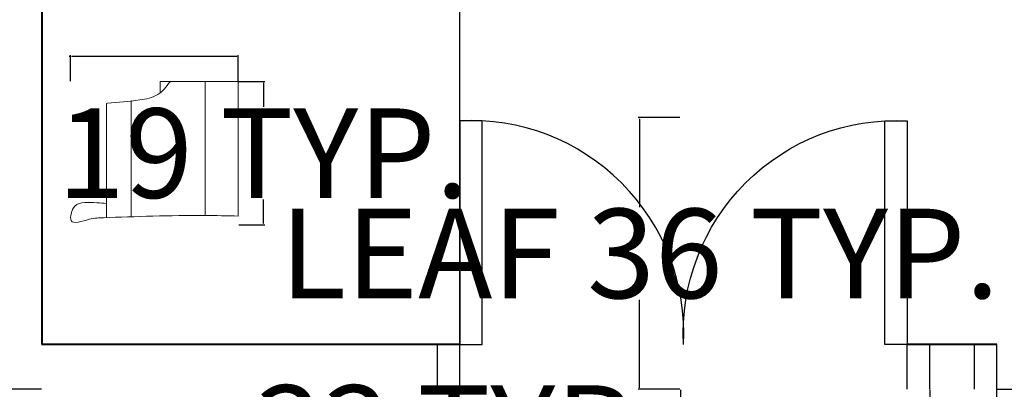
# Model space of a CAD drawing. Units: inches. Extents: x -124 to 612, y -69 to 524.
# Tile 3 of 9: x 16 to 148, y 190 to 240. Entities that reach past the tile are written whole.
import ezdxf

# ---------------------------------------------------------------- set-up
doc = ezdxf.new("R2010")
doc.units = ezdxf.units.IN
doc.header["$MEASUREMENT"] = 0
for name, color, linetype, lineweight in [('A-ANNO-DIMS', 2, 'Continuous', 18), ('A-DOOR', 4, 'Continuous', 25), ('A-FURN', 8, 'Continuous', 18), ('A-WALL', 7, 'Continuous', 40)]:
    doc.layers.add(name, color=color, linetype=linetype, lineweight=lineweight)
doc.styles.get("Standard").update_dxf_attribs({"font": 'arial.ttf'})
doc.dimstyles.get("Standard").update_dxf_attribs({"dimtxt": 12, "dimasz": 0.18, "dimexe": 0.18, "dimexo": 0.0625, "dimgap": 0.09, "dimtad": 0, "dimtih": 1, "dimtoh": 1, "dimdec": 0, "dimzin": 0, "dimdsep": 46, "dimlunit": 4, "dimtxsty": 'Standard', "dimcen": 0.09, "dimadec": 0, "dimazin": 0, "dimtfac": 1, "dimtdec": 0, "dimtofl": 0, "dimtmove": 0, "dimatfit": 3, "dimfxl": 1, "dimtolj": 1, "dimtzin": 0, "dimarcsym": 0})

# ---------------------------------------------------------------- blocks, each defined once
blk = doc.blocks.new('A$C43184A5C')
for p, q in [((723.6, 800), (29.6, 800)), ((724.2, 794.5), (723.6, 800.1)), ((740.3, 650), (34.6, 650)), ((855.9, 473.7), (788, 473.7)), ((855.9, 0), (855.9, 473.7)), ((855.9, 200), (42.4, 200)), ((39, 0.1), (39, 0)), ((855.9, 0), (39, 0))]:
    blk.add_line(p, q)
for points, knots in [([(116.1, 800), (117, 818.9), (119.9, 882), (130.6, 984.2), (58.7, 1017.3), (-22.2, 1023.5), (26.3, 904.6), (33.9, 661.4), (46.4, 338.8), (40.5, 67.6), (39, 0.1)], [4.965253, 4.965253, 4.965253, 4.965253, 63.558713, 198.678228, 250.994518, 291.108293, 401.549508, 488.981253, 1103.790728, 1307.592638, 1307.592638, 1307.592638, 1307.592638]), ([(854.7, 414.4), (825.5, 436.5), (764.7, 482.8), (737.2, 627.4), (729.3, 730.2), (724.3, 795.2)], [0, 0, 0, 0, 106.359769, 221.555283, 419.666547, 419.666547, 419.666547, 419.666547])]:
    blk.add_open_spline(points, degree=3, knots=knots)
blk = doc.blocks.new('DOOR-30IN-STAIR')
for p, q in [((0, 30.04), (0, 36.04)), ((3, 30.04), (3, 36.04)), ((33, 30.04), (33, 36.04)), ((36, 30.04), (36, 36.04))]:
    blk.add_line(p, q)
blk.add_lwpolyline([(3, 30.04), (6, 30.04), (6, 0.04), (3, 0.04)], close=True)
blk.add_arc((4.5, 28.54), 28.54, 266.9872, 3.0128)
blk = doc.blocks.new('DOOR-30IN-ENTRY-LEAF')
for p, q in [((0, 0), (0, 6)), ((3, 0), (3, 6))]:
    blk.add_line(p, q)
blk.add_lwpolyline([(3, 6), (6, 6), (6, 36), (3, 36)], close=True)
blk.add_arc((4.5, 7.5), 28.54, 356.9872, 93.0128)
blk = doc.blocks.new('*D27')
at = {"layer": 'A-ANNO-DIMS', "color": 0, "lineweight": -2, "transparency": 16777216}
for p, q in [((23.16, 234.66), (22.98, 234.66)), ((23.16, 231.34), (23.16, 234.84)), ((45.48, 234.66), (23.34, 234.66)), ((45.66, 231.34), (45.66, 234.84))]:
    blk.add_line(p, q, dxfattribs=at)
at = {"layer": 'A-ANNO-DIMS', "color": 0, "transparency": 16777216}
for points in [[(23.34, 234.69), (23.34, 234.63), (23.16, 234.66)], [(45.48, 234.69), (45.48, 234.63), (45.66, 234.66)]]:
    blk.add_solid(points, dxfattribs=at)
at = {"layer": 'Defpoints', "color": 0, "transparency": 16777216}
for p in [(23.16, 234.66), (23.16, 231.28), (45.66, 231.28)]:
    blk.add_point(p, dxfattribs=at)
at = {"layer": 'A-ANNO-DIMS', "color": 0, "transparency": 16777216, "insert": (-53.7, 234.66), "char_height": 12, "attachment_point": 5}
blk.add_mtext('\\A1;ARMCHAIR 23 TYP.', dxfattribs=at)
blk = doc.blocks.new('*D28')
at = {"layer": 'A-ANNO-DIMS', "color": 0, "lineweight": -2, "transparency": 16777216}
for p, q in [((45.72, 231.28), (49.21, 231.28)), ((49.03, 231.1), (49.03, 227.9)), ((49.03, 212.27), (49.03, 215.47)), ((45.72, 212.09), (49.21, 212.09))]:
    blk.add_line(p, q, dxfattribs=at)
at = {"layer": 'A-ANNO-DIMS', "color": 0, "transparency": 16777216}
for points in [[(49, 231.1), (49.06, 231.1), (49.03, 231.28)], [(49, 212.27), (49.06, 212.27), (49.03, 212.09)]]:
    blk.add_solid(points, dxfattribs=at)
at = {"layer": 'Defpoints', "color": 0, "transparency": 16777216}
for p in [(45.66, 231.28), (49.03, 231.28), (45.66, 212.09)]:
    blk.add_point(p, dxfattribs=at)
at = {"layer": 'A-ANNO-DIMS', "color": 0, "transparency": 16777216, "insert": (49.03, 221.69), "char_height": 12, "attachment_point": 5}
blk.add_mtext('\\A1;19 TYP.', dxfattribs=at)
blk = doc.blocks.new('*D39')
at = {"layer": 'A-ANNO-DIMS', "color": 0, "lineweight": -2, "transparency": 16777216}
for p, q in [((180.41, 196.03), (186, 196.03)), ((185.82, 195.85), (185.82, 184.12)), ((185.82, 159.78), (185.82, 171.51)), ((180.41, 159.6), (186, 159.6))]:
    blk.add_line(p, q, dxfattribs=at)
at = {"layer": 'A-ANNO-DIMS', "color": 0, "transparency": 16777216}
for points in [[(185.79, 195.85), (185.85, 195.85), (185.82, 196.03)], [(185.79, 159.78), (185.85, 159.78), (185.82, 159.6)]]:
    blk.add_solid(points, dxfattribs=at)
at = {"layer": 'Defpoints', "color": 0, "transparency": 16777216}
for p in [(180.35, 196.03), (185.82, 196.03), (180.35, 159.6)]:
    blk.add_point(p, dxfattribs=at)
at = {"layer": 'A-ANNO-DIMS', "color": 0, "transparency": 16777216, "insert": (185.82, 177.82), "char_height": 12, "attachment_point": 5}
blk.add_mtext('\\A1;STAIR DOOR 36 TYP.', dxfattribs=at)
blk = doc.blocks.new('*D41')
at = {"layer": 'A-ANNO-DIMS', "color": 0, "lineweight": -2, "transparency": 16777216}
for p, q in [((104.86, 226.45), (99.28, 226.45)), ((99.46, 226.27), (99.46, 214.46)), ((99.46, 190.21), (99.46, 202.02)), ((104.86, 190.03), (99.28, 190.03))]:
    blk.add_line(p, q, dxfattribs=at)
at = {"layer": 'A-ANNO-DIMS', "color": 0, "transparency": 16777216}
for points in [[(99.43, 226.27), (99.49, 226.27), (99.46, 226.45)], [(99.43, 190.21), (99.49, 190.21), (99.46, 190.03)]]:
    blk.add_solid(points, dxfattribs=at)
at = {"layer": 'Defpoints', "color": 0, "transparency": 16777216}
for p in [(99.46, 226.45), (104.93, 226.45), (104.93, 190.03)]:
    blk.add_point(p, dxfattribs=at)
at = {"layer": 'A-ANNO-DIMS', "color": 0, "transparency": 16777216, "insert": (99.46, 208.24), "char_height": 12, "attachment_point": 5}
blk.add_mtext('\\A1;LEAF 36 TYP.', dxfattribs=at)
blk = doc.blocks.new('*D42')
at = {"layer": 'A-ANNO-DIMS', "color": 0, "lineweight": -2, "transparency": 16777216}
for p, q in [((104.93, 189.97), (104.93, 184.39)), ((138.35, 189.97), (138.35, 184.39)), ((104.93, 184.57), (104.75, 184.57)), ((138.17, 184.57), (105.11, 184.57))]:
    blk.add_line(p, q, dxfattribs=at)
at = {"layer": 'A-ANNO-DIMS', "color": 0, "transparency": 16777216}
for points in [[(105.11, 184.6), (105.11, 184.54), (104.93, 184.57)], [(138.17, 184.6), (138.17, 184.54), (138.35, 184.57)]]:
    blk.add_solid(points, dxfattribs=at)
at = {"layer": 'Defpoints', "color": 0, "transparency": 16777216}
for p in [(104.93, 190.03), (138.35, 190.03), (104.93, 184.57)]:
    blk.add_point(p, dxfattribs=at)
at = {"layer": 'A-ANNO-DIMS', "color": 0, "transparency": 16777216, "insert": (75.45, 184.57), "char_height": 12, "attachment_point": 5}
blk.add_mtext('\\A1;33 TYP.', dxfattribs=at)
blk = doc.blocks.new('*D45')
at = {"layer": 'A-ANNO-DIMS', "color": 0, "lineweight": -2, "transparency": 16777216}
for p, q in [((142.74, 261.33), (142.74, 251.59)), ((206.86, 261.33), (206.86, 251.59)), ((142.92, 251.77), (206.68, 251.77)), ((206.86, 251.77), (207.04, 251.77))]:
    blk.add_line(p, q, dxfattribs=at)
at = {"layer": 'A-ANNO-DIMS', "color": 0, "transparency": 16777216}
for points in [[(142.92, 251.8), (142.92, 251.74), (142.74, 251.77)], [(206.68, 251.8), (206.68, 251.74), (206.86, 251.77)]]:
    blk.add_solid(points, dxfattribs=at)
at = {"layer": 'Defpoints', "color": 0, "transparency": 16777216}
for p in [(142.74, 261.39), (206.86, 261.39), (206.86, 251.77)]:
    blk.add_point(p, dxfattribs=at)
at = {"layer": 'A-ANNO-DIMS', "color": 0, "transparency": 16777216, "insert": (265.7, 251.77), "char_height": 12, "attachment_point": 5}
blk.add_mtext('\\A1;DINING SET 64', dxfattribs=at)
blk = doc.blocks.new('*D51')
at = {"layer": 'A-ANNO-DIMS', "color": 0, "lineweight": -2, "transparency": 16777216}
for p, q in [((19.35, 196.09), (19.35, 516.46)), ((19.53, 516.28), (38.67, 516.28)), ((75.17, 516.28), (56.03, 516.28)), ((75.35, 196.09), (75.35, 516.46))]:
    blk.add_line(p, q, dxfattribs=at)
at = {"layer": 'A-ANNO-DIMS', "color": 0, "transparency": 16777216}
for points in [[(19.53, 516.31), (19.53, 516.25), (19.35, 516.28)], [(75.17, 516.31), (75.17, 516.25), (75.35, 516.28)]]:
    blk.add_solid(points, dxfattribs=at)
at = {"layer": 'Defpoints', "color": 0, "transparency": 16777216}
for p in [(75.35, 516.28), (19.35, 196.03), (75.35, 196.03)]:
    blk.add_point(p, dxfattribs=at)
at = {"layer": 'A-ANNO-DIMS', "color": 0, "transparency": 16777216, "insert": (47.35, 516.28), "char_height": 12, "attachment_point": 5}
blk.add_mtext('\\A1;56', dxfattribs=at)
blk = doc.blocks.new('*D56')
at = {"layer": 'A-ANNO-DIMS', "color": 0, "lineweight": -2, "transparency": 16777216}
for p, q in [((19.29, 328.03), (-19.08, 328.03)), ((-18.9, 327.85), (-18.9, 265.25)), ((-18.9, 190.21), (-18.9, 252.81)), ((19.29, 190.03), (-19.08, 190.03))]:
    blk.add_line(p, q, dxfattribs=at)
at = {"layer": 'A-ANNO-DIMS', "color": 0, "transparency": 16777216}
for points in [[(-18.93, 327.85), (-18.87, 327.85), (-18.9, 328.03)], [(-18.93, 190.21), (-18.87, 190.21), (-18.9, 190.03)]]:
    blk.add_solid(points, dxfattribs=at)
at = {"layer": 'Defpoints', "color": 0, "transparency": 16777216}
for p in [(-18.9, 328.03), (19.35, 328.03), (19.35, 190.03)]:
    blk.add_point(p, dxfattribs=at)
at = {"layer": 'A-ANNO-DIMS', "color": 0, "transparency": 16777216, "insert": (-18.9, 259.03), "char_height": 12, "attachment_point": 5}
blk.add_mtext('\\A1;138', dxfattribs=at)

msp = doc.modelspace()

# ---------------------------------------------------------------- linework, layer by layer
at = {"layer": 'A-DOOR'}
for points in [[(75.3513, 196.0291), (78.3513, 196.0291), (78.3513, 226.0291), (75.3513, 226.0291)], [(135.3513, 196.0291), (132.3513, 196.0291), (132.3513, 226.0291), (135.3513, 226.0291)]]:
    msp.add_lwpolyline(points, close=True, dxfattribs=at)
msp.add_arc((76.8513, 197.5291), 28.5394, 356.987212, 93.012788, dxfattribs=at)
at = {"layer": 'A-WALL'}
for p, q in [((19.3513, 328.0291), (19.3513, 196.0291)), ((75.3513, 196.0291), (19.3513, 196.0291)), ((147.3513, 196.0291), (135.3513, 196.0291))]:
    msp.add_line(p, q, dxfattribs=at)

# ---------------------------------------------------------------- block references
at = {"layer": 'A-DOOR'}
for name, p in [('DOOR-30IN-ENTRY-LEAF', (72.351, 190.029)), ('DOOR-30IN-STAIR', (144.351, 159.99))]:
    msp.add_blockref(name, p, dxfattribs=at)
at = {"layer": 'A-DOOR', "extrusion": (0, 0, -1), "zscale": -1}
msp.add_blockref('DOOR-30IN-ENTRY-LEAF', (-138.3516, 190.029), dxfattribs=at)
at = {"layer": 'A-FURN', "xscale": 0.0220597728682114, "yscale": 0.0220597728682114, "zscale": 0.0220597728682114, "rotation": 90}
msp.add_blockref('A$C43184A5C', (45.6588, 212.4005), dxfattribs=at)

# ---------------------------------------------------------------- dimensions: what is measured, and where the dimension line sits
at = {"layer": 'A-ANNO-DIMS'}
dim = msp.add_linear_dim(base=(75.3513, 516.2791), p1=(19.3513, 196.0291), p2=(75.3513, 196.0291), dimstyle='Standard', override={"dimdec": 0, "dimlfac": 1, "dimrnd": 0, "dimzin": 0, "dimdsep": 46, "dimlunit": 2}, dxfattribs=at)
dim.commit()
dim.dimension.update_dxf_attribs({"geometry": '*D51', "text_midpoint": (47.3513, 516.2791)})
dim = msp.add_linear_dim(base=(-18.8987, 328.0291), p1=(19.3513, 190.0291), p2=(19.3513, 328.0291), angle=90, dimstyle='Standard', override={"dimdec": 0, "dimlfac": 1, "dimrnd": 0, "dimzin": 0, "dimdsep": 46, "dimlunit": 2}, dxfattribs=at)
dim.commit()
dim.dimension.update_dxf_attribs({"geometry": '*D56', "text_midpoint": (-18.8987, 259.0291)})
dim = msp.add_linear_dim(base=(206.8595, 251.775), p1=(142.7351, 261.3936), p2=(206.8595, 261.3936), text='DINING SET <>', dimstyle='Standard', override={"dimdec": 0, "dimlfac": 1, "dimrnd": 0, "dimzin": 0, "dimdsep": 46, "dimlunit": 2}, dxfattribs=at)
dim.commit()
dim.dimension.update_dxf_attribs({"geometry": '*D45', "text_midpoint": (265.697, 251.775)})
for base, p1, p2, angle, text, picture, middle in [((23.1554, 234.656), (45.6588, 231.2805), (23.1554, 231.2805), 180, 'ARMCHAIR <> TYP.', '*D27', (-53.7026, 234.656)), ((49.0343, 231.2805), (45.6588, 212.091), (45.6588, 231.2805), 90, '<> TYP.', '*D28', (49.0343, 221.6858)), ((99.4623, 226.4543), (104.9261, 190.0291), (104.9261, 226.4543), 90, 'LEAF <> TYP.', '*D41', (99.4623, 208.2417)), ((185.8151, 196.0291), (180.3513, 159.6038), (180.3513, 196.0291), 90, 'STAIR DOOR <> TYP.', '*D39', (185.8151, 177.8164)), ((104.9261, 184.5653), (138.3513, 190.0291), (104.9261, 190.0291), 180, '<> TYP.', '*D42', (75.4542, 184.5653))]:
    dim = msp.add_linear_dim(base=base, p1=p1, p2=p2, angle=angle, text=text, dimstyle='Standard', override={"dimdec": 0, "dimlfac": 1, "dimrnd": 0, "dimzin": 0, "dimdsep": 46, "dimlunit": 2}, dxfattribs=at)
    dim.commit()
    dim.dimension.update_dxf_attribs({"geometry": picture, "text_midpoint": middle})

doc.saveas('drawing.dxf')
